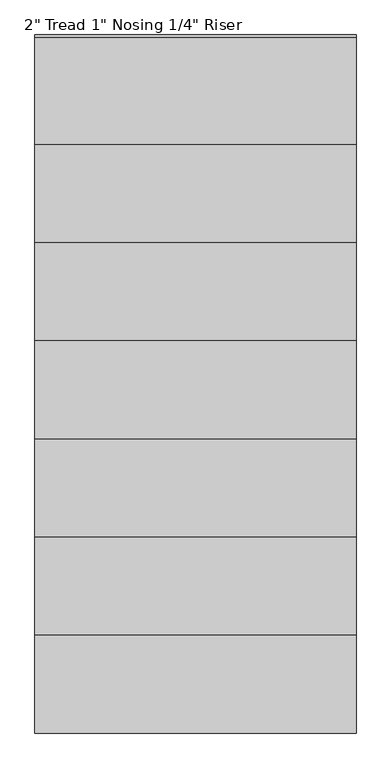
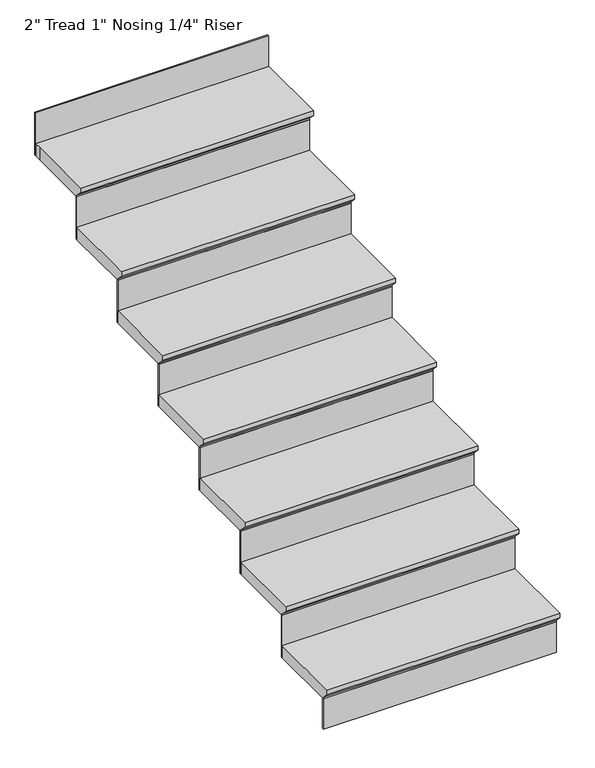
"""IFC4 building model written with IfcOpenShell, lengths in millimetres: stair flight geometry."""

from ifc_helpers import new_model, si_unit, origin, place, context, project, spatial, faceted_brep, source, transform, mapped, element, save


def stair_flight_e21d000d(model_context):
    return source(origin(), model_context, "Body", "Brep", [
        faceted_brep([(1046.3501403, 157.6257925, 7169.15), (1046.3501403, 157.6257925, 7188.2), (131.9501403, 157.6257925, 7188.2), (131.9501403, 157.6257925, 7169.15), (1046.3501403, 183.0257925, 7143.75), (131.9501403, 183.0257925, 7143.75), (1046.3501403, 462.4257925, 7188.2), (131.9501403, 462.4257925, 7188.2), (131.9501403, 183.0257925, 7137.4), (131.9501403, 462.4257925, 7137.4), (1046.3501403, 462.4257925, 7137.4), (1046.3501403, 183.0257925, 7137.4)], [[[0, 1, 2, 3]], [[4, 0, 3, 5]], [[2, 1, 6, 7]], [[8, 9, 10, 11]], [[2, 7, 9, 8, 5, 3]], [[8, 11, 4, 5]], [[6, 1, 0, 4, 11, 10]], [[7, 6, 10, 9]]]),
        faceted_brep([(1046.3501403, 183.0257925, 7137.4), (1046.3501403, 183.0257925, 7010.4), (1046.3501403, 189.3757925, 7010.4), (1046.3501403, 189.3757925, 7137.4), (131.9501403, 183.0257925, 7137.4), (131.9501403, 189.3757925, 7137.4), (131.9501403, 189.3757925, 7010.4), (131.9501403, 183.0257925, 7010.4)], [[[0, 1, 2, 3]], [[4, 5, 6, 7]], [[1, 0, 4, 7]], [[2, 1, 7, 6]], [[3, 2, 6, 5]], [[0, 3, 5, 4]]]),
        faceted_brep([(1046.3501403, 462.4257925, 7315.2), (1046.3501403, 462.4257925, 7137.4), (1046.3501403, 468.7757925, 7137.4), (1046.3501403, 468.7757925, 7315.2), (131.9501403, 462.4257925, 7315.2), (131.9501403, 468.7757925, 7315.2), (131.9501403, 468.7757925, 7137.4), (131.9501403, 462.4257925, 7137.4)], [[[0, 1, 2, 3]], [[4, 5, 6, 7]], [[1, 0, 4, 7]], [[2, 1, 7, 6]], [[3, 2, 6, 5]], [[0, 3, 5, 4]]]),
        faceted_brep([(131.9501403, 437.0257925, 7366.0), (1046.3501403, 437.0257925, 7366.0), (1046.3501403, 741.8257925, 7366.0), (131.9501403, 741.8257925, 7366.0), (131.9501403, 462.4257925, 7315.2), (131.9501403, 741.8257925, 7315.2), (1046.3501403, 741.8257925, 7315.2), (1046.3501403, 462.4257925, 7315.2), (131.9501403, 462.4257925, 7321.55), (131.9501403, 437.0257925, 7346.95), (1046.3501403, 462.4257925, 7321.55), (1046.3501403, 437.0257925, 7346.95)], [[[0, 1, 2, 3]], [[4, 5, 6, 7]], [[0, 3, 5, 4, 8, 9]], [[4, 7, 10, 8]], [[2, 1, 11, 10, 7, 6]], [[3, 2, 6, 5]], [[11, 1, 0, 9]], [[10, 11, 9, 8]]]),
        faceted_brep([(1046.3501403, 741.8257925, 7493.0), (1046.3501403, 741.8257925, 7315.2), (1046.3501403, 748.1757925, 7315.2), (1046.3501403, 748.1757925, 7493.0), (131.9501403, 741.8257925, 7493.0), (131.9501403, 748.1757925, 7493.0), (131.9501403, 748.1757925, 7315.2), (131.9501403, 741.8257925, 7315.2)], [[[0, 1, 2, 3]], [[4, 5, 6, 7]], [[1, 0, 4, 7]], [[2, 1, 7, 6]], [[3, 2, 6, 5]], [[0, 3, 5, 4]]]),
        faceted_brep([(131.9501403, 716.4257925, 7543.8), (1046.3501403, 716.4257925, 7543.8), (1046.3501403, 1021.2257925, 7543.8), (131.9501403, 1021.2257925, 7543.8), (131.9501403, 741.8257925, 7493.0), (131.9501403, 1021.2257925, 7493.0), (1046.3501403, 1021.2257925, 7493.0), (1046.3501403, 741.8257925, 7493.0), (131.9501403, 741.8257925, 7499.35), (131.9501403, 716.4257925, 7524.75), (1046.3501403, 741.8257925, 7499.35), (1046.3501403, 716.4257925, 7524.75)], [[[0, 1, 2, 3]], [[4, 5, 6, 7]], [[0, 3, 5, 4, 8, 9]], [[4, 7, 10, 8]], [[2, 1, 11, 10, 7, 6]], [[3, 2, 6, 5]], [[11, 1, 0, 9]], [[10, 11, 9, 8]]]),
        faceted_brep([(1046.3501403, 1021.2257925, 7670.8), (1046.3501403, 1021.2257925, 7493.0), (1046.3501403, 1027.5757925, 7493.0), (1046.3501403, 1027.5757925, 7670.8), (131.9501403, 1021.2257925, 7670.8), (131.9501403, 1027.5757925, 7670.8), (131.9501403, 1027.5757925, 7493.0), (131.9501403, 1021.2257925, 7493.0)], [[[0, 1, 2, 3]], [[4, 5, 6, 7]], [[1, 0, 4, 7]], [[2, 1, 7, 6]], [[3, 2, 6, 5]], [[0, 3, 5, 4]]]),
        faceted_brep([(131.9501403, 995.8257925, 7721.6), (1046.3501403, 995.8257925, 7721.6), (1046.3501403, 1300.6257925, 7721.6), (131.9501403, 1300.6257925, 7721.6), (131.9501403, 1021.2257925, 7670.8), (131.9501403, 1300.6257925, 7670.8), (1046.3501403, 1300.6257925, 7670.8), (1046.3501403, 1021.2257925, 7670.8), (131.9501403, 1021.2257925, 7677.15), (131.9501403, 995.8257925, 7702.55), (1046.3501403, 1021.2257925, 7677.15), (1046.3501403, 995.8257925, 7702.55)], [[[0, 1, 2, 3]], [[4, 5, 6, 7]], [[0, 3, 5, 4, 8, 9]], [[4, 7, 10, 8]], [[2, 1, 11, 10, 7, 6]], [[3, 2, 6, 5]], [[11, 1, 0, 9]], [[10, 11, 9, 8]]]),
        faceted_brep([(1046.3501403, 1300.6257925, 7848.6), (1046.3501403, 1300.6257925, 7670.8), (1046.3501403, 1306.9757925, 7670.8), (1046.3501403, 1306.9757925, 7848.6), (131.9501403, 1300.6257925, 7848.6), (131.9501403, 1306.9757925, 7848.6), (131.9501403, 1306.9757925, 7670.8), (131.9501403, 1300.6257925, 7670.8)], [[[0, 1, 2, 3]], [[4, 5, 6, 7]], [[1, 0, 4, 7]], [[2, 1, 7, 6]], [[3, 2, 6, 5]], [[0, 3, 5, 4]]]),
        faceted_brep([(131.9501403, 1275.2257925, 7899.4), (1046.3501403, 1275.2257925, 7899.4), (1046.3501403, 1580.0257925, 7899.4), (131.9501403, 1580.0257925, 7899.4), (131.9501403, 1300.6257925, 7848.6), (131.9501403, 1580.0257925, 7848.6), (1046.3501403, 1580.0257925, 7848.6), (1046.3501403, 1300.6257925, 7848.6), (131.9501403, 1300.6257925, 7854.95), (131.9501403, 1275.2257925, 7880.35), (1046.3501403, 1300.6257925, 7854.95), (1046.3501403, 1275.2257925, 7880.35)], [[[0, 1, 2, 3]], [[4, 5, 6, 7]], [[0, 3, 5, 4, 8, 9]], [[4, 7, 10, 8]], [[2, 1, 11, 10, 7, 6]], [[3, 2, 6, 5]], [[11, 1, 0, 9]], [[10, 11, 9, 8]]]),
        faceted_brep([(1046.3501403, 1580.0257925, 8026.4), (1046.3501403, 1580.0257925, 7848.6), (1046.3501403, 1586.3757925, 7848.6), (1046.3501403, 1586.3757925, 8026.4), (131.9501403, 1580.0257925, 8026.4), (131.9501403, 1586.3757925, 8026.4), (131.9501403, 1586.3757925, 7848.6), (131.9501403, 1580.0257925, 7848.6)], [[[0, 1, 2, 3]], [[4, 5, 6, 7]], [[1, 0, 4, 7]], [[2, 1, 7, 6]], [[3, 2, 6, 5]], [[0, 3, 5, 4]]]),
        faceted_brep([(131.9501403, 1554.6257925, 8077.2), (1046.3501403, 1554.6257925, 8077.2), (1046.3501403, 1859.4257925, 8077.2), (131.9501403, 1859.4257925, 8077.2), (131.9501403, 1580.0257925, 8026.4), (131.9501403, 1859.4257925, 8026.4), (1046.3501403, 1859.4257925, 8026.4), (1046.3501403, 1580.0257925, 8026.4), (131.9501403, 1580.0257925, 8032.75), (131.9501403, 1554.6257925, 8058.15), (1046.3501403, 1580.0257925, 8032.75), (1046.3501403, 1554.6257925, 8058.15)], [[[0, 1, 2, 3]], [[4, 5, 6, 7]], [[0, 3, 5, 4, 8, 9]], [[4, 7, 10, 8]], [[2, 1, 11, 10, 7, 6]], [[3, 2, 6, 5]], [[11, 1, 0, 9]], [[10, 11, 9, 8]]]),
        faceted_brep([(1046.3501403, 2138.8257925, 8382.0), (1046.3501403, 2138.8257925, 8204.2), (1046.3501403, 2145.1757925, 8204.2), (1046.3501403, 2145.1757925, 8382.0), (131.9501403, 2138.8257925, 8382.0), (131.9501403, 2145.1757925, 8382.0), (131.9501403, 2145.1757925, 8204.2), (131.9501403, 2138.8257925, 8204.2)], [[[0, 1, 2, 3]], [[4, 5, 6, 7]], [[1, 0, 4, 7]], [[2, 1, 7, 6]], [[3, 2, 6, 5]], [[0, 3, 5, 4]]]),
        faceted_brep([(1046.3501403, 1859.4257925, 8204.2), (1046.3501403, 1859.4257925, 8026.4), (1046.3501403, 1865.7757925, 8026.4), (1046.3501403, 1865.7757925, 8204.2), (131.9501403, 1859.4257925, 8204.2), (131.9501403, 1865.7757925, 8204.2), (131.9501403, 1865.7757925, 8026.4), (131.9501403, 1859.4257925, 8026.4)], [[[0, 1, 2, 3]], [[4, 5, 6, 7]], [[1, 0, 4, 7]], [[2, 1, 7, 6]], [[3, 2, 6, 5]], [[0, 3, 5, 4]]]),
        faceted_brep([(131.9501403, 2138.8257925, 8255.0), (131.9501403, 2113.4257925, 8255.0), (131.9501403, 1834.0257925, 8255.0), (1046.3501403, 1834.0257925, 8255.0), (1046.3501403, 2138.8257925, 8255.0), (131.9501403, 2113.4257925, 8204.2), (131.9501403, 2138.8257925, 8204.2), (1046.3501403, 2138.8257925, 8204.2), (1046.3501403, 1859.4257925, 8204.2), (131.9501403, 1859.4257925, 8204.2), (131.9501403, 1859.4257925, 8210.55), (131.9501403, 1834.0257925, 8235.95), (1046.3501403, 1859.4257925, 8210.55), (1046.3501403, 1834.0257925, 8235.95)], [[[0, 1, 2, 3, 4]], [[5, 6, 7, 8, 9]], [[1, 0, 6, 5]], [[2, 1, 5, 9, 10, 11]], [[9, 8, 12, 10]], [[4, 3, 13, 12, 8, 7]], [[0, 4, 7, 6]], [[13, 3, 2, 11]], [[12, 13, 11, 10]]]),
    ])


if __name__ == "__main__":
    model = new_model("IFC4")
    model_context = context("Model", 3, world=origin())
    ifc_project = project(units=[si_unit("LENGTHUNIT", "METRE", prefix="MILLI")], contexts=[model_context])
    site = spatial("IfcSite", under=ifc_project)
    building = spatial("IfcBuilding", under=site)
    placement = place(None, origin())
    stair_flight_shape = stair_flight_e21d000d(model_context)
    element("IfcStairFlight", 1, ObjectType="2\" Tread 1\" Nosing 1/4\" Riser", at=placement, inside=building, context=model_context, shape_type="MappedRepresentation", body=[
        mapped(stair_flight_shape, transform((0.0, 0.0, 0.0), x_axis=(1.0, 0.0, 0.0), y_axis=(0.0, 1.0, 0.0), z_axis=(0.0, 0.0, 1.0))),
    ])
    save(model, "model.ifc")
